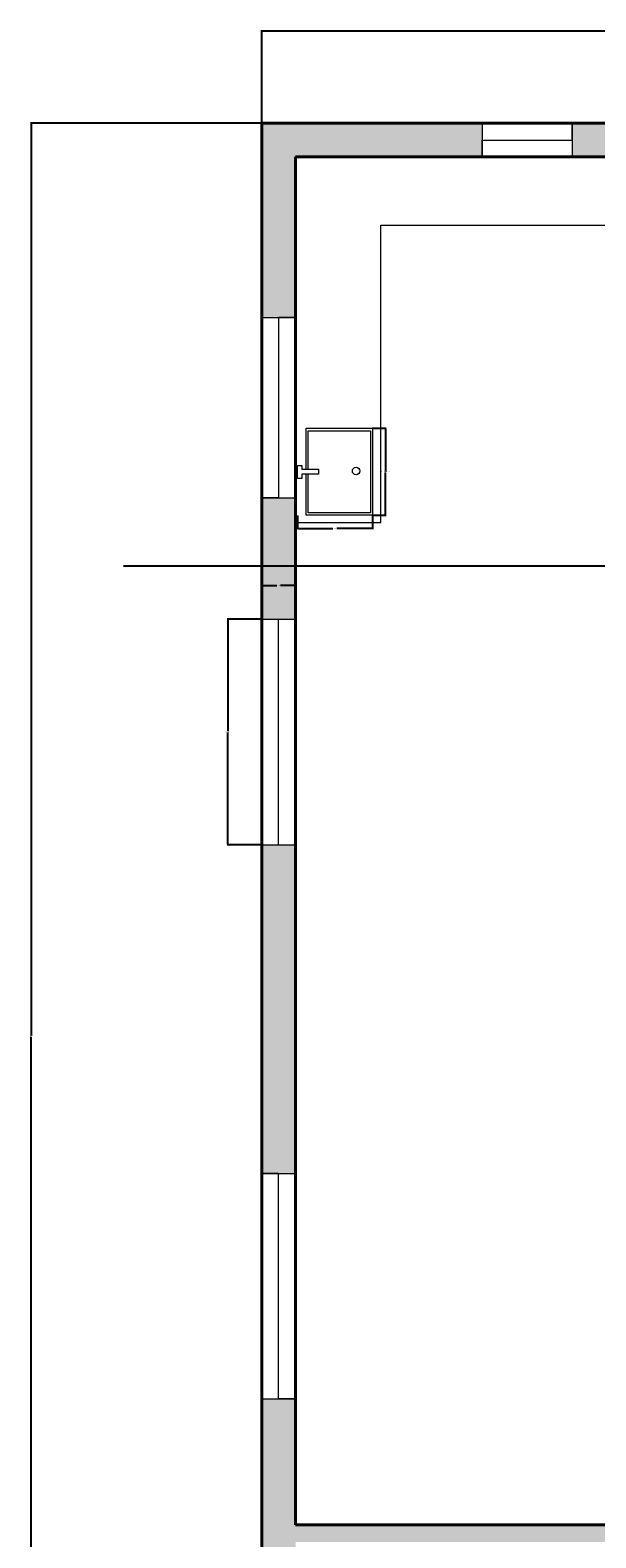
# Model space of a CAD drawing. Units: inches. Extents: x 1441 to 2460, y 1648 to 2683.
# Tile 31 of 35: x 1976 to 2127, y 1922 to 2323. Entities that reach past the tile are written whole.
import ezdxf

# ---------------------------------------------------------------- set-up
doc = ezdxf.new("R2010")
doc.units = ezdxf.units.IN
for name, color, linetype, lineweight in [('A-ANNO-DIMS', 2, 'Continuous', 18), ('A-ANNO-SYMB', 5, 'Continuous', 25), ('A-FLOR-CASE', 9, 'Continuous', 20), ('A-FLOR-FIXT', 9, 'Continuous', 18), ('A-GLAZ', 4, 'Continuous', 18), ('A-WALL', 7, 'Continuous', 40)]:
    doc.layers.add(name, color=color, linetype=linetype, lineweight=lineweight)
doc.layers.add('A-WALL-PATT', color=251, linetype='Continuous', lineweight=13, true_color=0x636466)
doc.styles.get("Standard").update_dxf_attribs({"font": 'arial.ttf'})
doc.dimstyles.get("Standard").update_dxf_attribs({"dimtxt": 0.18, "dimasz": 0.18, "dimexe": 0.18, "dimexo": 0.0625, "dimgap": 0.09, "dimtad": 0, "dimtih": 1, "dimtoh": 1, "dimdec": 4, "dimzin": 0, "dimdsep": 46, "dimtxsty": 'Standard', "dimcen": 0.09, "dimadec": 0, "dimazin": 0, "dimtfac": 1, "dimtdec": 4, "dimtofl": 0, "dimtmove": 0, "dimatfit": 3, "dimfxl": 1, "dimtolj": 1, "dimtzin": 0, "dimarcsym": 0})

# ---------------------------------------------------------------- blocks, each defined once
blk = doc.blocks.new('WIN-48-SASH')
for p, q in [((9, 48), (4.5, 48)), ((4.5, 48), (4.5, 0)), ((4.5, 0), (0, 0))]:
    blk.add_line(p, q)
blk = doc.blocks.new('WIN-60-SASH')
for p, q in [((9, 60), (4.5, 60)), ((4.5, 60), (4.5, 0)), ((4.5, 0), (0, 0))]:
    blk.add_line(p, q)
blk = doc.blocks.new('SINK-KITCHEN')
for points in [[(2.36, 12.29), (2.36, 23.19), (19.96, 23.19), (19.96, 0), (2.36, 0), (2.36, 10.91)], [(2.84, 12.29), (2.84, 22.51), (19.43, 22.51), (19.43, 0.62), (2.84, 0.62), (2.84, 10.91)], [(1.21, 10.91), (1.21, 9.78), (0, 9.78), (0, 13.22), (1.21, 13.22), (1.21, 12.29)], [(1.21, 12.29), (5.65, 12.29), (5.65, 10.91), (1.21, 10.91)]]:
    blk.add_lwpolyline(points)
blk.add_circle((15.62, 11.79), 0.997)
blk = doc.blocks.new('*D36')
at = {"layer": 'A-ANNO-DIMS', "color": 0, "lineweight": -2, "transparency": 16777216}
for p, q in [((2067.42, 2217.53), (2071.02, 2217.53)), ((2070.84, 2217.35), (2070.84, 2206.12)), ((2070.84, 2194.52), (2070.84, 2205.75)), ((2067.42, 2194.34), (2071.02, 2194.34))]:
    blk.add_line(p, q, dxfattribs=at)
at = {"layer": 'A-ANNO-DIMS', "color": 0, "transparency": 16777216}
for points in [[(2070.81, 2217.35), (2070.87, 2217.35), (2070.84, 2217.53)], [(2070.81, 2194.52), (2070.87, 2194.52), (2070.84, 2194.34)]]:
    blk.add_solid(points, dxfattribs=at)
at = {"layer": 'Defpoints', "color": 0, "transparency": 16777216}
for p in [(2067.36, 2217.53), (2070.84, 2217.53), (2067.36, 2194.34)]:
    blk.add_point(p, dxfattribs=at)
at = {"layer": 'A-ANNO-DIMS', "color": 0, "transparency": 16777216, "insert": (2070.84, 2205.93), "char_height": 0.18, "attachment_point": 5}
blk.add_mtext('\\A1;KITCHEN SINK 23 TYP.', dxfattribs=at)
blk = doc.blocks.new('*D37')
at = {"layer": 'A-ANNO-DIMS', "color": 0, "lineweight": -2, "transparency": 16777216}
for p, q in [((2047.39, 2194.27), (2047.39, 2190.68)), ((2047.57, 2190.86), (2056.84, 2190.86)), ((2067.18, 2190.86), (2057.9, 2190.86)), ((2067.36, 2194.27), (2067.36, 2190.68))]:
    blk.add_line(p, q, dxfattribs=at)
at = {"layer": 'A-ANNO-DIMS', "color": 0, "transparency": 16777216}
for points in [[(2047.57, 2190.89), (2047.57, 2190.83), (2047.39, 2190.86)], [(2067.18, 2190.89), (2067.18, 2190.83), (2067.36, 2190.86)]]:
    blk.add_solid(points, dxfattribs=at)
at = {"layer": 'Defpoints', "color": 0, "transparency": 16777216}
for p in [(2047.39, 2194.34), (2067.36, 2194.34), (2067.36, 2190.86)]:
    blk.add_point(p, dxfattribs=at)
at = {"layer": 'A-ANNO-DIMS', "color": 0, "transparency": 16777216, "insert": (2057.37, 2190.86), "char_height": 0.18, "attachment_point": 5}
blk.add_mtext('\\A1;20 TYP.', dxfattribs=at)
blk = doc.blocks.new('*D62')
at = {"layer": 'A-ANNO-DIMS', "color": 0, "lineweight": -2, "transparency": 16777216}
for p, q in [((2037.84, 2166.69), (2028.72, 2166.69)), ((2028.9, 2166.51), (2028.9, 2136.87)), ((2028.9, 2106.87), (2028.9, 2136.51)), ((2037.84, 2106.69), (2028.72, 2106.69))]:
    blk.add_line(p, q, dxfattribs=at)
at = {"layer": 'A-ANNO-DIMS', "color": 0, "transparency": 16777216}
for points in [[(2028.87, 2166.51), (2028.93, 2166.51), (2028.9, 2166.69)], [(2028.87, 2106.87), (2028.93, 2106.87), (2028.9, 2106.69)]]:
    blk.add_solid(points, dxfattribs=at)
at = {"layer": 'Defpoints', "color": 0, "transparency": 16777216}
for p in [(2037.9, 2166.69), (2028.9, 2106.69), (2037.9, 2106.69)]:
    blk.add_point(p, dxfattribs=at)
at = {"layer": 'A-ANNO-DIMS', "color": 0, "transparency": 16777216, "insert": (2028.9, 2136.69), "char_height": 0.18, "attachment_point": 5}
blk.add_mtext('\\A1;SASH 60 TYP.', dxfattribs=at)
blk = doc.blocks.new('*D63')
at = {"layer": 'A-ANNO-DIMS', "color": 0, "lineweight": -2, "transparency": 16777216}
for p, q in [((2037.9, 2166.75), (2037.9, 2175.87)), ((2038.08, 2175.69), (2041.94, 2175.69)), ((2046.72, 2175.69), (2042.86, 2175.69)), ((2046.9, 2166.75), (2046.9, 2175.87))]:
    blk.add_line(p, q, dxfattribs=at)
at = {"layer": 'A-ANNO-DIMS', "color": 0, "transparency": 16777216}
for points in [[(2038.08, 2175.72), (2038.08, 2175.66), (2037.9, 2175.69)], [(2046.72, 2175.72), (2046.72, 2175.66), (2046.9, 2175.69)]]:
    blk.add_solid(points, dxfattribs=at)
at = {"layer": 'Defpoints', "color": 0, "transparency": 16777216}
for p in [(2037.9, 2175.69), (2037.9, 2166.69), (2046.9, 2166.69)]:
    blk.add_point(p, dxfattribs=at)
at = {"layer": 'A-ANNO-DIMS', "color": 0, "transparency": 16777216, "insert": (2042.4, 2175.69), "char_height": 0.18, "attachment_point": 5}
blk.add_mtext('\\A1;9 TYP.', dxfattribs=at)
blk = doc.blocks.new('*D80')
at = {"layer": 'A-ANNO-DIMS', "color": 0, "lineweight": -2, "transparency": 16777216}
for p, q in [((2037.9, 2298.76), (2037.9, 2323.43)), ((2038.08, 2323.25), (2197.76, 2323.25)), ((2358.22, 2323.25), (2198.55, 2323.25)), ((2358.4, 2298.76), (2358.4, 2323.43))]:
    blk.add_line(p, q, dxfattribs=at)
at = {"layer": 'A-ANNO-DIMS', "color": 0, "transparency": 16777216}
for points in [[(2038.08, 2323.28), (2038.08, 2323.22), (2037.9, 2323.25)], [(2358.22, 2323.28), (2358.22, 2323.22), (2358.4, 2323.25)]]:
    blk.add_solid(points, dxfattribs=at)
at = {"layer": 'Defpoints', "color": 0, "transparency": 16777216}
for p in [(2358.4, 2323.25), (2037.9, 2298.7), (2358.4, 2298.7)]:
    blk.add_point(p, dxfattribs=at)
at = {"layer": 'A-ANNO-DIMS', "color": 0, "transparency": 16777216, "insert": (2198.15, 2323.25), "char_height": 0.18, "attachment_point": 5}
blk.add_mtext('\\A1;320.5', dxfattribs=at)
blk = doc.blocks.new('*D81')
at = {"layer": 'A-ANNO-DIMS', "color": 0, "lineweight": -2, "transparency": 16777216}
for p, q in [((2037.84, 2298.7), (1976.42, 2298.7)), ((1976.6, 2298.52), (1976.6, 2055.94)), ((1976.6, 1813), (1976.6, 2055.57)), ((2154.24, 1812.82), (1976.42, 1812.82))]:
    blk.add_line(p, q, dxfattribs=at)
at = {"layer": 'A-ANNO-DIMS', "color": 0, "transparency": 16777216}
for points in [[(1976.57, 2298.52), (1976.63, 2298.52), (1976.6, 2298.7)], [(1976.57, 1813), (1976.63, 1813), (1976.6, 1812.82)]]:
    blk.add_solid(points, dxfattribs=at)
at = {"layer": 'Defpoints', "color": 0, "transparency": 16777216}
for p in [(1976.6, 2298.7), (2037.9, 2298.7), (2154.3, 1812.82)]:
    blk.add_point(p, dxfattribs=at)
at = {"layer": 'A-ANNO-DIMS', "color": 0, "transparency": 16777216, "insert": (1976.6, 2055.76), "char_height": 0.18, "attachment_point": 5}
blk.add_mtext('\\A1;485.9', dxfattribs=at)

msp = doc.modelspace()

# ---------------------------------------------------------------- hatches: boundary and pattern name
at = {"layer": 'A-WALL-PATT'}
h = msp.add_hatch(color=256, dxfattribs=at)
h.dxf.hatch_style = 1
h.paths.add_polyline_path([(2096.524, 2298.6952), (2037.9015, 2298.6952), (2037.9015, 2246.9605), (2046.9015, 2246.9605), (2046.9015, 2289.6952), (2096.524, 2289.6952), (2096.524, 2294.1952)])
h.paths.add_polyline_path([(2144.5933, 2298.6952), (2120.524, 2298.6952), (2120.524, 2289.6952), (2144.5933, 2289.6952), (2144.5933, 2294.1952)])
h.paths.add_polyline_path([(2136.4015, 2289.6952), (2131.9015, 2289.6952), (2131.9015, 2233.0622), (2136.4015, 2233.0622)])
h.paths.add_polyline_path([(2184.8877, 2294.3362), (2184.8877, 2295.2788), (2184.8877, 2298.6952), (2168.5933, 2298.6952), (2168.5933, 2289.6952), (2184.8877, 2289.6952)])
h.paths.add_polyline_path([(2176.9015, 2289.6952), (2172.4015, 2289.6952), (2172.4015, 2199.6952), (2176.9015, 2199.6952)])
h.paths.add_polyline_path([(2229.4015, 2204.637), (2224.9015, 2204.637), (2224.9015, 2199.6952), (2136.4015, 2199.6952), (2136.4015, 2204.637), (2131.9015, 2204.637), (2131.9015, 2195.1952), (2229.4015, 2195.1952)])
h.paths.add_polyline_path([(2229.4015, 2289.6952), (2224.9015, 2289.6952), (2224.9015, 2233.0622), (2229.4015, 2233.0622)])
h.paths.add_polyline_path([(2358.4015, 2298.6952), (2208.8877, 2298.6952), (2208.8877, 2289.6952), (2349.4015, 2289.6952), (2349.4015, 2250.8051), (2358.4015, 2250.8051)])
h.paths.add_polyline_path([(2358.4015, 2202.8051), (2349.4015, 2202.8051), (2349.4015, 2157.6952), (2216.9636, 2157.6952), (2216.9636, 2153.1952), (2224.9015, 2153.1952), (2224.9015, 2058.005), (2229.4015, 2058.005), (2229.4015, 2153.1952), (2349.4015, 2153.1952), (2349.4015, 2124.108), (2358.4015, 2124.108)])
h.paths.add_polyline_path([(2358.4015, 1984.8305), (2349.4015, 1984.8305), (2349.4015, 1834.1952), (2358.4015, 1834.1952)])
h.paths.add_polyline_path([(2358.4015, 2076.108), (2349.4015, 2076.108), (2349.4015, 2008.8305), (2358.4015, 2008.8305)])
h.paths.add_polyline_path([(2349.4015, 2027.1952), (2269.9015, 2027.1952), (2269.9015, 2000.9452), (2274.4015, 2000.9452), (2274.4015, 2022.6952), (2349.4015, 2022.6952)])
h.paths.add_polyline_path([(2269.9015, 2027.1952), (2229.4015, 2027.1952), (2229.4015, 2030.7912), (2224.9015, 2030.7912), (2224.9015, 2022.6952), (2269.9015, 2022.6952)])
h.paths.add_polyline_path([(2349.4015, 1974.6952), (2274.4015, 1974.6952), (2274.4015, 1978.7973), (2269.9015, 1978.7973), (2269.9015, 1974.6952), (2263.8979, 1974.6952), (2263.8979, 1970.1952), (2269.9015, 1970.1952), (2274.4015, 1970.1952), (2349.4015, 1970.1952)])
h.paths.add_polyline_path([(2229.4015, 1974.6952), (2224.9015, 1974.6952), (2224.9015, 1925.6952), (2220.8772, 1925.6952), (2220.8772, 1921.1952), (2229.4015, 1921.1952)])
h.paths.add_polyline_path([(2229.4015, 1921.1952), (2224.9015, 1921.1952), (2224.9015, 1843.1952), (2229.4015, 1843.1952)])
h.paths.add_polyline_path([(2268.1291, 1838.6952), (2268.1291, 1843.1952), (2229.4015, 1843.1952), (2220.91, 1843.1952), (2220.91, 1834.1952), (2227.1771, 1834.1952), (2268.1291, 1834.1952)])
h.paths.add_polyline_path([(2349.4015, 1843.1952), (2328.1291, 1843.1952), (2328.1291, 1834.1952), (2349.4015, 1834.1952)])
h.paths.add_polyline_path([(2046.9015, 1857.7914), (2037.9015, 1857.7914), (2037.9015, 1834.1952), (2164.019, 1834.1952), (2164.019, 1838.6952), (2164.019, 1843.1952), (2046.9015, 1843.1952)])
h.paths.add_polyline_path([(2046.9015, 1959.2399), (2042.4015, 1959.2399), (2037.9015, 1959.2399), (2037.9015, 1905.7914), (2046.9015, 1905.7914), (2046.9015, 1921.1952), (2172.4015, 1921.1952), (2176.9015, 1921.1952), (2184.1657, 1921.1952), (2184.1657, 1925.6952), (2176.9015, 1925.6952), (2172.4015, 1925.6952), (2046.9015, 1925.6952)])
h.paths.add_polyline_path([(2046.9015, 2106.6907), (2037.9015, 2106.6907), (2037.9015, 2019.2399), (2046.9015, 2019.2399)])
h.paths.add_polyline_path([(2176.9015, 2051.6952), (2172.4015, 2051.6952), (2172.4015, 2048.6952), (2172.4015, 1925.6952), (2176.9015, 1925.6952)])
h.paths.add_polyline_path([(2172.4015, 2051.6952), (2145.4015, 2051.6952), (2145.4015, 2048.6952), (2172.4015, 2048.6952)])
h.paths.add_polyline_path([(2172.4015, 2102.6952), (2145.4015, 2102.6952), (2145.4015, 2099.6952), (2154.4015, 2099.6952), (2172.4015, 2099.6952)])
h.paths.add_polyline_path([(2176.9015, 2153.1952), (2179.5767, 2153.1952), (2179.5767, 2157.6952), (2176.9015, 2157.6952), (2176.9015, 2195.1952), (2172.4015, 2195.1952), (2172.4015, 2099.6952), (2176.9015, 2099.6952)])
h.paths.add_polyline_path([(2046.9015, 2198.9605), (2037.9015, 2198.9605), (2037.9015, 2166.6907), (2046.9015, 2166.6907)])

# ---------------------------------------------------------------- linework, layer by layer
at = {"layer": 'A-ANNO-SYMB'}
msp.add_line((2001.1539, 2180.8746), (2395.889, 2180.8746), dxfattribs=at)
at = {"layer": 'A-FLOR-CASE'}
for p, q in [((2069.5886, 2192.432), (2069.5886, 2271.5733)), ((2069.5886, 2271.5733), (2131.9015, 2271.5733)), ((2046.9015, 2192.432), (2053.8762, 2192.432)), ((2053.8762, 2192.432), (2069.5886, 2192.432))]:
    msp.add_line(p, q, dxfattribs=at)
at = {"layer": 'A-GLAZ'}
for p, q in [((2096.524, 2298.6952), (2096.524, 2289.6952)), ((2120.524, 2294.1952), (2120.524, 2298.6952)), ((2120.524, 2298.6952), (2120.524, 2289.6952)), ((2096.524, 2289.6952), (2096.524, 2294.1952)), ((2096.524, 2294.1952), (2120.524, 2294.1952)), ((2037.9015, 2246.9605), (2046.9015, 2246.9605)), ((2037.9015, 2198.9605), (2046.9015, 2198.9605)), ((2037.9015, 2166.6907), (2046.9015, 2166.6907)), ((2037.9015, 2106.6907), (2046.9015, 2106.6907)), ((2042.4015, 2019.2399), (2037.9015, 2019.2399)), ((2037.9015, 2019.2399), (2046.9015, 2019.2399)), ((2042.4015, 1959.2399), (2042.4015, 2019.2399)), ((2037.9015, 1959.2399), (2046.9015, 1959.2399)), ((2046.9015, 1959.2399), (2042.4015, 1959.2399))]:
    msp.add_line(p, q, dxfattribs=at)
at = {"layer": 'A-WALL'}
for p, q in [((2037.9015, 2298.6952), (2037.9015, 1834.1952)), ((2037.9015, 2298.6952), (2358.4015, 2298.6952)), ((2046.9015, 2289.6952), (2046.9015, 2157.6952)), ((2046.9015, 2289.6952), (2046.9015, 1925.6952)), ((2046.9015, 2289.6952), (2349.4015, 2289.6952)), ((2172.4015, 1925.6952), (2046.9015, 1925.6952))]:
    msp.add_line(p, q, dxfattribs=at)

# ---------------------------------------------------------------- block references
at = {"layer": 'A-FLOR-FIXT'}
msp.add_blockref('SINK-KITCHEN', (2047.3956, 2194.34), dxfattribs=at)
at = {"layer": 'A-GLAZ'}
msp.add_blockref('WIN-48-SASH', (2037.9056, 2198.96), dxfattribs=at)
at = {"layer": 'A-GLAZ', "rotation": 180}
msp.add_blockref('WIN-60-SASH', (2046.8974, 2166.6914), dxfattribs=at)

# ---------------------------------------------------------------- dimensions: what is measured, and where the dimension line sits
at = {"layer": 'A-ANNO-DIMS'}
dim = msp.add_linear_dim(base=(2358.4015, 2323.2452), p1=(2037.9015, 2298.6952), p2=(2358.4015, 2298.6952), dimstyle='Standard', override={"dimdec": 1, "dimlfac": 1, "dimrnd": 0, "dimzin": 0, "dimdsep": 46, "dimlunit": 2}, dxfattribs=at)
dim.commit()
dim.dimension.update_dxf_attribs({"geometry": '*D80', "text_midpoint": (2198.1515, 2323.2452)})
dim = msp.add_linear_dim(base=(1976.6039, 2298.6952), p1=(2154.3041, 1812.8171), p2=(2037.9015, 2298.6952), angle=90, dimstyle='Standard', override={"dimdec": 1, "dimlfac": 1, "dimrnd": 0, "dimzin": 0, "dimdsep": 46, "dimlunit": 2}, dxfattribs=at)
dim.commit()
dim.dimension.update_dxf_attribs({"geometry": '*D81', "text_midpoint": (1976.6039, 2055.7561)})
for base, p1, p2, angle, text, picture, middle in [((2070.8376, 2217.5321), (2067.3583, 2194.3371), (2067.3583, 2217.5321), 90, 'KITCHEN SINK <> TYP.', '*D36', (2070.8376, 2205.9346)), ((2037.9015, 2175.6907), (2046.9015, 2166.6907), (2037.9015, 2166.6907), 180, '<> TYP.', '*D63', (2042.4015, 2175.6907)), ((2028.9015, 2106.6907), (2037.9015, 2166.6907), (2037.9015, 2106.6907), 270, 'SASH <> TYP.', '*D62', (2028.9015, 2136.6907))]:
    dim = msp.add_linear_dim(base=base, p1=p1, p2=p2, angle=angle, text=text, dimstyle='Standard', override={"dimdec": 0, "dimlfac": 1, "dimrnd": 0, "dimzin": 0, "dimdsep": 46, "dimlunit": 2}, dxfattribs=at)
    dim.commit()
    dim.dimension.update_dxf_attribs({"geometry": picture, "text_midpoint": middle})
dim = msp.add_linear_dim(base=(2067.3583, 2190.8578), p1=(2047.3906, 2194.3371), p2=(2067.3583, 2194.3371), text='<> TYP.', dimstyle='Standard', override={"dimdec": 0, "dimlfac": 1, "dimrnd": 0, "dimzin": 0, "dimdsep": 46, "dimlunit": 2}, dxfattribs=at)
dim.commit()
dim.dimension.update_dxf_attribs({"geometry": '*D37', "text_midpoint": (2057.3745, 2190.8578)})

doc.saveas('drawing.dxf')
